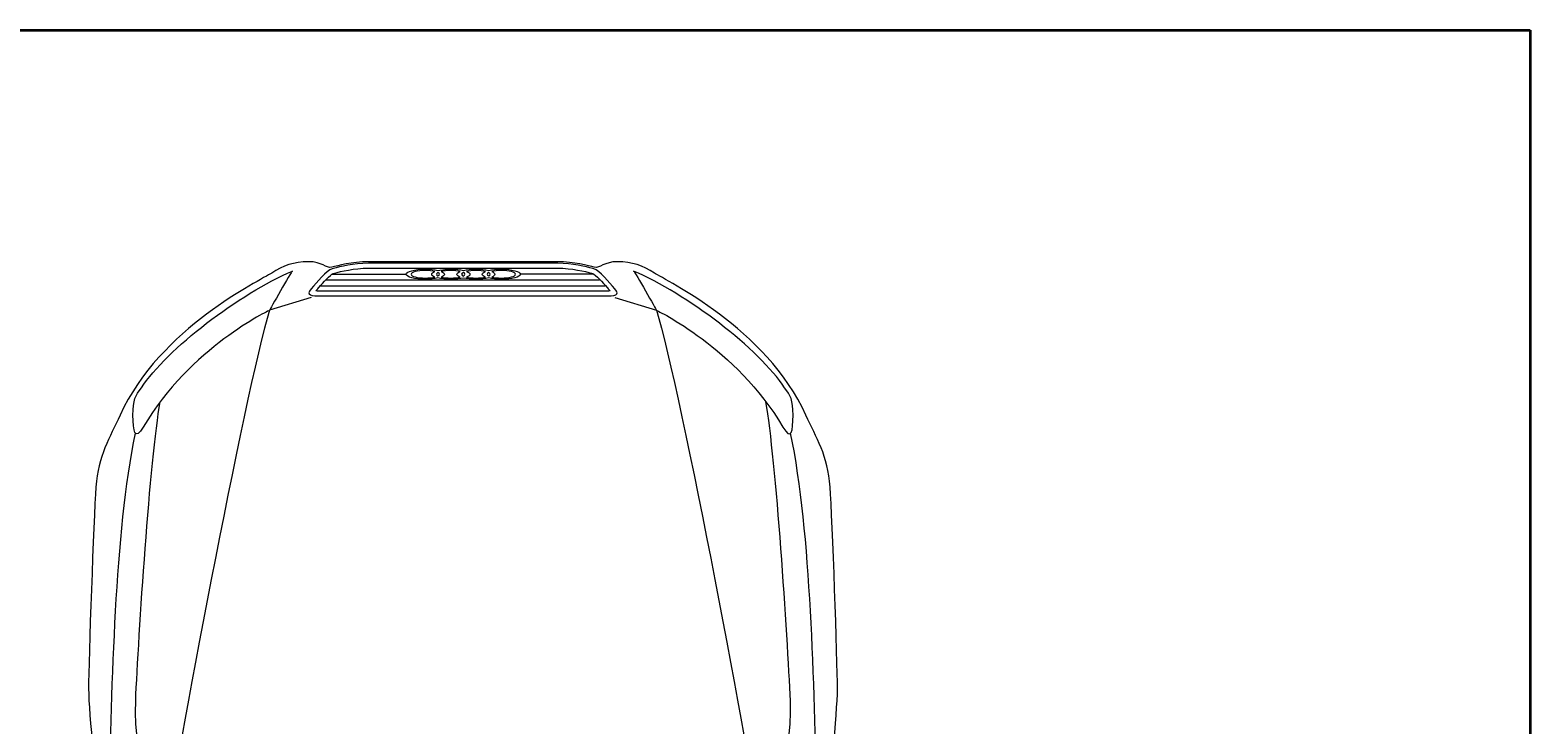
# Model space of a CAD drawing. Units: inches. Extents: x 1911 to 3278, y 2022 to 3108.
# Tile 5 of 13: x 2045 to 2118, y 2230 to 2264. Entities that reach past the tile are written whole.
import ezdxf

# ---------------------------------------------------------------- set-up
doc = ezdxf.new("R2010")
doc.units = ezdxf.units.IN
for name, color, linetype, lineweight in [('A-ANNO-DIMS', 2, 'Continuous', 18), ('A-WALL', 7, 'Continuous', 35), ('AUDI', 7, 'Continuous', 18)]:
    doc.layers.add(name, color=color, linetype=linetype, lineweight=lineweight)
doc.styles.get("Standard").update_dxf_attribs({"font": 'arial.ttf'})
doc.dimstyles.get("Standard").update_dxf_attribs({"dimtxt": 0.18, "dimasz": 0.18, "dimexe": 0.18, "dimexo": 0.0625, "dimgap": 0.09, "dimtad": 0, "dimtih": 1, "dimtoh": 1, "dimdec": 4, "dimzin": 0, "dimdsep": 46, "dimtxsty": 'Standard', "dimcen": 0.09, "dimadec": 0, "dimazin": 0, "dimtfac": 1, "dimtdec": 4, "dimtofl": 0, "dimtmove": 0, "dimatfit": 3, "dimfxl": 1, "dimtolj": 1, "dimtzin": 0, "dimarcsym": 0})

# ---------------------------------------------------------------- blocks, each defined once
blk = doc.blocks.new('*D68')
at = {"layer": 'A-ANNO-DIMS', "color": 0, "lineweight": -2, "transparency": 16777216}
for p, q in [((2016.834, 2263.811), (2016.834, 2048.124)), ((2117.834, 2263.811), (2117.834, 2048.124)), ((2017.014, 2048.304), (2067.071, 2048.304)), ((2117.654, 2048.304), (2067.597, 2048.304))]:
    blk.add_line(p, q, dxfattribs=at)
at = {"layer": 'A-ANNO-DIMS', "color": 0, "transparency": 16777216}
for points in [[(2017.014, 2048.334), (2017.014, 2048.274), (2016.834, 2048.304)], [(2117.654, 2048.334), (2117.654, 2048.274), (2117.834, 2048.304)]]:
    blk.add_solid(points, dxfattribs=at)
at = {"layer": 'Defpoints', "color": 0, "transparency": 16777216}
for p in [(2016.834, 2263.873), (2117.834, 2263.873), (2117.834, 2048.304)]:
    blk.add_point(p, dxfattribs=at)
at = {"layer": 'A-ANNO-DIMS', "color": 0, "transparency": 16777216, "insert": (2067.334, 2048.304), "char_height": 0.18, "attachment_point": 5}
blk.add_mtext('\\A1;101', dxfattribs=at)

msp = doc.modelspace()

# ---------------------------------------------------------------- linework, layer by layer
at = {"layer": 'A-WALL'}
for p, q in [((2016.8344, 2263.8733), (2117.8344, 2263.8733)), ((2117.8344, 2263.8733), (2117.8344, 2217.8733))]:
    msp.add_line(p, q, dxfattribs=at)
at = {"layer": 'AUDI'}
for points, knots in [([(2065.7636, 2161.2036), (2052.3657, 2161.35), (2050.4204, 2165.8553), (2049.5983, 2168.8238), (2049.5983, 2168.8238), (2049.0621, 2170.5764), (2048.6333, 2171.9712), (2048.4187, 2172.6866), (2048.4187, 2172.6866), (2048.2042, 2173.4019), (2047.7397, 2175.5836), (2047.7038, 2177.4077), (2047.7038, 2177.4077), (2047.6679, 2179.2318), (2047.491, 2190.1075), (2047.491, 2193.1091), (2047.491, 2193.1091), (2047.491, 2196.1105), (2047.491, 2210.1722), (2047.491, 2212.1725), (2047.491, 2212.1725), (2047.491, 2214.1727), (2047.9184, 2222.1512), (2047.9184, 2224.6905), (2047.9184, 2224.6905), (2047.9184, 2227.23), (2047.491, 2230.416), (2047.491, 2231.7362), (2047.491, 2231.7362), (2047.491, 2233.0566), (2047.7395, 2240.034), (2047.8468, 2241.572), (2047.8468, 2241.572), (2047.9542, 2243.11), (2048.5301, 2243.9822), (2049.0266, 2245.0771), (2049.0266, 2245.0771), (2050.9569, 2249.333), (2055.8898, 2251.6577), (2056.426, 2252.0154), (2056.426, 2252.0154), (2056.9622, 2252.3732), (2057.5315, 2252.5675), (2058.2133, 2252.5675), (2058.2133, 2252.5675), (2058.8952, 2252.5675), (2059.0712, 2252.2302), (2059.3573, 2252.3017), (2059.3573, 2252.3017), (2059.6432, 2252.3732), (2060.3558, 2252.5675), (2061.1448, 2252.5675), (2061.1448, 2252.5675), (2061.9338, 2252.5675), (2065.7636, 2252.5675), (2065.7636, 2252.5675), (2065.7636, 2252.5675), (2065.7636, 2252.5675), (2069.5936, 2252.5675), (2070.3825, 2252.5675), (2070.3825, 2252.5675), (2071.1717, 2252.5675), (2071.8841, 2252.3732), (2072.1701, 2252.3017), (2072.1701, 2252.3017), (2072.4561, 2252.2302), (2072.6322, 2252.5675), (2073.314, 2252.5675), (2073.314, 2252.5675), (2073.9959, 2252.5675), (2074.5651, 2252.3732), (2075.1013, 2252.0154), (2075.1013, 2252.0154), (2075.6375, 2251.6577), (2080.5704, 2249.333), (2082.5007, 2245.0771), (2082.5007, 2245.0771), (2082.9972, 2243.9822), (2083.5731, 2243.1099), (2083.6805, 2241.572), (2083.6805, 2241.572), (2083.7879, 2240.0341), (2084.0364, 2233.0565), (2084.0364, 2231.7362), (2084.0364, 2231.7362), (2084.0364, 2230.4161), (2083.609, 2227.23), (2083.609, 2224.6905), (2083.609, 2224.6905), (2083.609, 2222.1512), (2084.0364, 2214.1727), (2084.0364, 2212.1725), (2084.0364, 2212.1725), (2084.0364, 2210.1722), (2084.0364, 2196.1105), (2084.0364, 2193.1091), (2084.0364, 2193.1091), (2084.0364, 2190.1075), (2083.8594, 2179.2318), (2083.8235, 2177.4077), (2083.8235, 2177.4077), (2083.7877, 2175.5836), (2083.3232, 2173.4019), (2083.1086, 2172.6866), (2083.1086, 2172.6866), (2082.8941, 2171.9712), (2082.4652, 2170.5764), (2081.9291, 2168.8238), (2081.9291, 2168.8238), (2081.107, 2165.8553), (2079.1616, 2161.35), (2065.7636, 2161.2036)], [0, 0, 0, 0, 0.0357143, 0.0357143, 0.0357143, 0.0357143, 0.0714286, 0.0714286, 0.0714286, 0.0714286, 0.1071429, 0.1071429, 0.1071429, 0.1071429, 0.1428571, 0.1428571, 0.1428571, 0.1428572, 0.1785714, 0.1785714, 0.1785714, 0.1785714, 0.2142857, 0.2142857, 0.2142857, 0.2142857, 0.25, 0.25, 0.25, 0.25, 0.2857143, 0.2857143, 0.2857143, 0.2857143, 0.3214286, 0.3214286, 0.3214286, 0.3214286, 0.3571429, 0.3571429, 0.3571429, 0.3571429, 0.3928571, 0.3928571, 0.3928571, 0.3928572, 0.4285714, 0.4285714, 0.4285714, 0.4285714, 0.4642857, 0.4642857, 0.4642857, 0.4642857, 0.5, 0.5, 0.5, 0.5, 0.5357143, 0.5357143, 0.5357143, 0.5357143, 0.5714286, 0.5714286, 0.5714286, 0.5714286, 0.6071429, 0.6071429, 0.6071429, 0.6071429, 0.6428571, 0.6428571, 0.6428571, 0.6428572, 0.6785714, 0.6785714, 0.6785714, 0.6785714, 0.7142857, 0.7142857, 0.7142857, 0.7142857, 0.75, 0.75, 0.75, 0.75, 0.7857143, 0.7857143, 0.7857143, 0.7857143, 0.8214286, 0.8214286, 0.8214286, 0.8214286, 0.8571429, 0.8571429, 0.8571429, 0.8571429, 0.8928571, 0.8928571, 0.8928571, 0.8928572, 0.9285714, 0.9285714, 0.9285714, 0.9285714, 0.9642857, 0.9642857, 0.9642857, 0.9642857, 1, 1, 1, 1]), ([(2065.8389, 2252.4894), (2065.8389, 2252.4894), (2070.3825, 2252.4894), (2070.3825, 2252.4894), (2070.3825, 2252.4894), (2071.1113, 2252.4894), (2071.7728, 2252.3216), (2072.0906, 2252.2412), (2072.0906, 2252.2412), (2072.0906, 2252.2412), (2072.1511, 2252.2259), (2072.1511, 2252.2259), (2072.1511, 2252.2259), (2072.44, 2252.1337), (2072.887, 2251.5522), (2073.1702, 2251.2391), (2073.1702, 2251.2391), (2073.4534, 2250.9259), (2073.1702, 2250.8962), (2072.6635, 2250.8962), (2072.6635, 2250.8962), (2072.1568, 2250.8962), (2065.7636, 2250.8962), (2065.7636, 2250.8962), (2065.7636, 2250.8962), (2065.7636, 2250.8962), (2059.3705, 2250.8962), (2058.8638, 2250.8962), (2058.8638, 2250.8962), (2058.3572, 2250.8962), (2058.074, 2250.9259), (2058.3572, 2251.2391), (2058.3572, 2251.2391), (2058.6403, 2251.5522), (2059.0873, 2252.1336), (2059.3762, 2252.2259), (2059.3762, 2252.2259), (2059.3762, 2252.2259), (2059.4367, 2252.2412), (2059.4367, 2252.2412), (2059.4367, 2252.2412), (2059.7545, 2252.3216), (2060.416, 2252.4893), (2061.1448, 2252.4893), (2061.1448, 2252.4893), (2061.1448, 2252.4893), (2065.6885, 2252.4894), (2065.6885, 2252.4894), (2065.6885, 2252.4894), (2065.6885, 2252.4894), (2065.8389, 2252.4894), (2065.8389, 2252.4894)], [0, 0, 0, 0, 0.0769231, 0.0769231, 0.0769231, 0.0769231, 0.1538462, 0.1538462, 0.1538462, 0.1538462, 0.2307692, 0.2307692, 0.2307692, 0.2307692, 0.3076923, 0.3076923, 0.3076923, 0.3076923, 0.3846154, 0.3846154, 0.3846154, 0.3846154, 0.4615385, 0.4615385, 0.4615385, 0.4615385, 0.5384615, 0.5384615, 0.5384615, 0.5384615, 0.6153846, 0.6153846, 0.6153846, 0.6153846, 0.6923077, 0.6923077, 0.6923077, 0.6923077, 0.7692308, 0.7692308, 0.7692308, 0.7692308, 0.8461538, 0.8461538, 0.8461538, 0.8461539, 0.9230769, 0.9230769, 0.9230769, 0.9230769, 1, 1, 1, 1]), ([(2049.6568, 2245.0859), (2049.6568, 2244.2903), (2049.748, 2243.8077), (2050.1559, 2244.4983), (2050.1559, 2244.4983), (2052.4466, 2248.3769), (2056.3231, 2250.1984), (2056.3231, 2250.1984), (2056.3231, 2250.1984), (2056.3231, 2250.1984), (2057.3734, 2252.0821), (2057.4391, 2252.1083), (2057.4391, 2252.1083), (2054.8815, 2251.0258), (2051.2895, 2248.298), (2050.0679, 2246.4083), (2050.0679, 2246.4083), (2049.7743, 2246.0263), (2049.6568, 2245.8358), (2049.6568, 2245.0859)], [0, 0, 0, 0, 0.2, 0.2, 0.2, 0.2, 0.4, 0.4, 0.4, 0.4, 0.6, 0.6, 0.6, 0.6, 0.8, 0.8, 0.8, 0.8, 1, 1, 1, 1]), ([(2049.6568, 2245.0859), (2049.6568, 2244.2903), (2049.748, 2243.8077), (2050.1559, 2244.4983), (2050.1559, 2244.4983), (2052.4466, 2248.3769), (2056.3231, 2250.1984), (2056.3231, 2250.1984), (2056.3231, 2250.1984), (2056.3231, 2250.1984), (2057.3734, 2252.0821), (2057.4391, 2252.1083), (2057.4391, 2252.1083), (2054.8815, 2251.0258), (2051.2895, 2248.298), (2050.0679, 2246.4083), (2050.0679, 2246.4083), (2049.7743, 2246.0263), (2049.6568, 2245.8358), (2049.6568, 2245.0859)], [0, 0, 0, 0, 0.2, 0.2, 0.2, 0.2, 0.4, 0.4, 0.4, 0.4, 0.6, 0.6, 0.6, 0.6, 0.8, 0.8, 0.8, 0.8, 1, 1, 1, 1]), ([(2058.8638, 2251.1329), (2058.8638, 2251.1329), (2058.8638, 2251.1329), (2058.8638, 2251.1329), (2058.8638, 2251.1329), (2058.8638, 2251.1329), (2072.6635, 2251.1329), (2072.6635, 2251.1329), (2072.6635, 2251.1329), (2072.78, 2251.1329), (2072.8697, 2251.1357), (2072.9424, 2251.1402), (2072.9424, 2251.1402), (2072.8866, 2251.2042), (2072.8004, 2251.3028), (2072.8004, 2251.3028), (2072.8004, 2251.3028), (2072.593, 2251.5439), (2072.2461, 2251.9466), (2072.0796, 2252), (2072.0796, 2252), (2072.0796, 2252), (2072.0328, 2252.0116), (2072.0328, 2252.0116), (2072.0328, 2252.0116), (2071.7231, 2252.0901), (2071.0812, 2252.2528), (2070.3825, 2252.2528), (2070.3825, 2252.2528), (2070.3825, 2252.2528), (2061.1448, 2252.2528), (2061.1448, 2252.2528), (2061.1448, 2252.2528), (2060.4462, 2252.2528), (2059.8043, 2252.09), (2059.4956, 2252.012), (2059.4956, 2252.012), (2059.4956, 2252.012), (2059.4341, 2251.9963), (2059.4341, 2251.9963), (2059.4341, 2251.9963), (2059.2817, 2251.9474), (2058.9346, 2251.5438), (2058.7269, 2251.3028), (2058.7269, 2251.3028), (2058.7269, 2251.3028), (2058.641, 2251.2042), (2058.585, 2251.1402), (2058.585, 2251.1402), (2058.6579, 2251.1358), (2058.7473, 2251.1329), (2058.8638, 2251.1329)], [0, 0, 0, 0, 0.0769231, 0.0769231, 0.0769231, 0.0769231, 0.1538462, 0.1538462, 0.1538462, 0.1538462, 0.2307692, 0.2307692, 0.2307692, 0.2307692, 0.3076923, 0.3076923, 0.3076923, 0.3076923, 0.3846154, 0.3846154, 0.3846154, 0.3846154, 0.4615385, 0.4615385, 0.4615385, 0.4615385, 0.5384615, 0.5384615, 0.5384615, 0.5384615, 0.6153846, 0.6153846, 0.6153846, 0.6153846, 0.6923077, 0.6923077, 0.6923077, 0.6923077, 0.7692308, 0.7692308, 0.7692308, 0.7692308, 0.8461538, 0.8461538, 0.8461538, 0.8461539, 0.9230769, 0.9230769, 0.9230769, 0.9230769, 1, 1, 1, 1]), ([(2063.921, 2251.7091), (2064.1614, 2251.7091), (2064.3716, 2251.7333), (2064.5366, 2251.7741), (2064.5366, 2251.7741), (2064.702, 2251.7333), (2064.9274, 2251.7091), (2065.1678, 2251.7091), (2065.1678, 2251.7091), (2065.4079, 2251.7091), (2065.6182, 2251.7333), (2065.7835, 2251.77), (2065.7835, 2251.77), (2065.9334, 2251.7333), (2066.1591, 2251.7091), (2066.3842, 2251.7091), (2066.3842, 2251.7091), (2066.6247, 2251.7091), (2066.85, 2251.7333), (2067.0152, 2251.7741), (2067.0152, 2251.7741), (2067.1804, 2251.7333), (2067.3906, 2251.7091), (2067.6309, 2251.7091), (2067.6309, 2251.7091), (2068.1418, 2251.7091), (2068.5623, 2251.8185), (2068.5623, 2251.956), (2068.5623, 2251.956), (2068.5623, 2252.0894), (2068.1418, 2252.2031), (2067.6309, 2252.2031), (2067.6309, 2252.2031), (2067.3906, 2252.2031), (2067.1804, 2252.1748), (2067.0152, 2252.1381), (2067.0152, 2252.1381), (2066.85, 2252.1748), (2066.6247, 2252.2031), (2066.3842, 2252.2031), (2066.3842, 2252.2031), (2066.1591, 2252.2031), (2065.9334, 2252.1788), (2065.7835, 2252.1381), (2065.7835, 2252.1381), (2065.6182, 2252.1789), (2065.4079, 2252.2031), (2065.1678, 2252.2031), (2065.1678, 2252.2031), (2064.9001, 2252.2031), (2064.6104, 2252.1546), (2064.5366, 2252.1381), (2064.5366, 2252.1381), (2064.3716, 2252.1748), (2064.1614, 2252.2031), (2063.921, 2252.2031), (2063.921, 2252.2031), (2063.4102, 2252.2031), (2062.9895, 2252.0894), (2062.9895, 2251.956), (2062.9895, 2251.956), (2062.9895, 2251.8185), (2063.4102, 2251.7091), (2063.921, 2251.7091)], [0, 0, 0, 0, 0.0625, 0.0625, 0.0625, 0.0625, 0.125, 0.125, 0.125, 0.125, 0.1875, 0.1875, 0.1875, 0.1875, 0.25, 0.25, 0.25, 0.25, 0.3125, 0.3125, 0.3125, 0.3125, 0.375, 0.375, 0.375, 0.375, 0.4375, 0.4375, 0.4375, 0.4375, 0.5, 0.5, 0.5, 0.5, 0.5625, 0.5625, 0.5625, 0.5625, 0.625, 0.625, 0.625, 0.625, 0.6875, 0.6875, 0.6875, 0.6875, 0.75, 0.75, 0.75, 0.75, 0.8125, 0.8125, 0.8125, 0.8125, 0.875, 0.875, 0.875, 0.875, 0.9375, 0.9375, 0.9375, 0.9375, 1, 1, 1, 1]), ([(2063.921, 2251.7091), (2064.1614, 2251.7091), (2064.3716, 2251.7333), (2064.5366, 2251.7741), (2064.5366, 2251.7741), (2064.702, 2251.7333), (2064.9274, 2251.7091), (2065.1678, 2251.7091), (2065.1678, 2251.7091), (2065.4079, 2251.7091), (2065.6182, 2251.7333), (2065.7835, 2251.77), (2065.7835, 2251.77), (2065.9334, 2251.7333), (2066.1591, 2251.7091), (2066.3842, 2251.7091), (2066.3842, 2251.7091), (2066.6247, 2251.7091), (2066.85, 2251.7333), (2067.0152, 2251.7741), (2067.0152, 2251.7741), (2067.1804, 2251.7333), (2067.3906, 2251.7091), (2067.6309, 2251.7091), (2067.6309, 2251.7091), (2068.1418, 2251.7091), (2068.5623, 2251.8185), (2068.5623, 2251.956), (2068.5623, 2251.956), (2068.5623, 2252.0894), (2068.1418, 2252.2031), (2067.6309, 2252.2031), (2067.6309, 2252.2031), (2067.3906, 2252.2031), (2067.1804, 2252.1748), (2067.0152, 2252.1381), (2067.0152, 2252.1381), (2066.85, 2252.1748), (2066.6247, 2252.2031), (2066.3842, 2252.2031), (2066.3842, 2252.2031), (2066.1591, 2252.2031), (2065.9334, 2252.1788), (2065.7835, 2252.1381), (2065.7835, 2252.1381), (2065.6182, 2252.1789), (2065.4079, 2252.2031), (2065.1678, 2252.2031), (2065.1678, 2252.2031), (2064.9001, 2252.2031), (2064.6104, 2252.1546), (2064.5366, 2252.1381), (2064.5366, 2252.1381), (2064.3716, 2252.1748), (2064.1614, 2252.2031), (2063.921, 2252.2031), (2063.921, 2252.2031), (2063.4102, 2252.2031), (2062.9895, 2252.0894), (2062.9895, 2251.956), (2062.9895, 2251.956), (2062.9895, 2251.8185), (2063.4102, 2251.7091), (2063.921, 2251.7091)], [0, 0, 0, 0, 0.0625, 0.0625, 0.0625, 0.0625, 0.125, 0.125, 0.125, 0.125, 0.1875, 0.1875, 0.1875, 0.1875, 0.25, 0.25, 0.25, 0.25, 0.3125, 0.3125, 0.3125, 0.3125, 0.375, 0.375, 0.375, 0.375, 0.4375, 0.4375, 0.4375, 0.4375, 0.5, 0.5, 0.5, 0.5, 0.5625, 0.5625, 0.5625, 0.5625, 0.625, 0.625, 0.625, 0.625, 0.6875, 0.6875, 0.6875, 0.6875, 0.75, 0.75, 0.75, 0.75, 0.8125, 0.8125, 0.8125, 0.8125, 0.875, 0.875, 0.875, 0.875, 0.9375, 0.9375, 0.9375, 0.9375, 1, 1, 1, 1]), ([(2063.921, 2252.1381), (2064.1011, 2252.1381), (2064.2665, 2252.122), (2064.3867, 2252.0894), (2064.3867, 2252.0894), (2064.2964, 2252.0491), (2064.2363, 2252.0046), (2064.2363, 2251.956), (2064.2363, 2251.956), (2064.2363, 2251.9034), (2064.2964, 2251.859), (2064.3867, 2251.8185), (2064.3867, 2251.8185), (2064.2665, 2251.7901), (2064.1011, 2251.77), (2063.921, 2251.77), (2063.921, 2251.77), (2063.5304, 2251.77), (2063.2299, 2251.8508), (2063.2299, 2251.956), (2063.2299, 2251.956), (2063.2299, 2252.0572), (2063.5304, 2252.1381), (2063.921, 2252.1381)], [0, 0, 0, 0, 0.1666667, 0.1666667, 0.1666667, 0.1666667, 0.3333333, 0.3333333, 0.3333333, 0.3333333, 0.5, 0.5, 0.5, 0.5, 0.6666667, 0.6666667, 0.6666667, 0.6666667, 0.8333333, 0.8333333, 0.8333333, 0.8333333, 1, 1, 1, 1]), ([(2064.612, 2251.956), (2064.612, 2251.9236), (2064.5819, 2251.8993), (2064.5366, 2251.8751), (2064.5366, 2251.8751), (2064.4918, 2251.8994), (2064.4767, 2251.9235), (2064.4767, 2251.956), (2064.4767, 2251.956), (2064.4767, 2251.9845), (2064.4918, 2252.0126), (2064.5366, 2252.037), (2064.5366, 2252.037), (2064.5819, 2252.0126), (2064.612, 2251.9845), (2064.612, 2251.956)], [0, 0, 0, 0, 0.25, 0.25, 0.25, 0.25, 0.5, 0.5, 0.5, 0.5, 0.75, 0.75, 0.75, 0.75, 1, 1, 1, 1]), ([(2065.6182, 2252.0935), (2065.5279, 2252.0532), (2065.4681, 2252.0046), (2065.4681, 2251.956), (2065.4681, 2251.956), (2065.4681, 2251.9034), (2065.5279, 2251.8549), (2065.6182, 2251.8144), (2065.6182, 2251.8144), (2065.4982, 2251.7861), (2065.3479, 2251.77), (2065.1678, 2251.77), (2065.1678, 2251.77), (2064.9873, 2251.77), (2064.8223, 2251.7901), (2064.702, 2251.8185), (2064.702, 2251.8185), (2064.7921, 2251.859), (2064.8522, 2251.9034), (2064.8522, 2251.956), (2064.8522, 2251.956), (2064.8522, 2252.0047), (2064.7921, 2252.0491), (2064.702, 2252.0894), (2064.702, 2252.0894), (2064.8223, 2252.1221), (2064.9873, 2252.1381), (2065.1678, 2252.1381), (2065.1678, 2252.1381), (2065.3479, 2252.1381), (2065.4982, 2252.122), (2065.6182, 2252.0935)], [0, 0, 0, 0, 0.125, 0.125, 0.125, 0.125, 0.25, 0.25, 0.25, 0.25, 0.375, 0.375, 0.375, 0.375, 0.5, 0.5, 0.5, 0.5, 0.625, 0.625, 0.625, 0.625, 0.75, 0.75, 0.75, 0.75, 0.875, 0.875, 0.875, 0.875, 1, 1, 1, 1]), ([(2065.8584, 2251.956), (2065.8584, 2251.9236), (2065.8286, 2251.8952), (2065.7835, 2251.8669), (2065.7835, 2251.8669), (2065.7233, 2251.8953), (2065.6934, 2251.9235), (2065.6934, 2251.956), (2065.6934, 2251.956), (2065.6934, 2251.9845), (2065.7233, 2252.0167), (2065.7835, 2252.0411), (2065.7835, 2252.0411), (2065.8286, 2252.0167), (2065.8584, 2251.9845), (2065.8584, 2251.956)], [0, 0, 0, 0, 0.25, 0.25, 0.25, 0.25, 0.5, 0.5, 0.5, 0.5, 0.75, 0.75, 0.75, 0.75, 1, 1, 1, 1]), ([(2066.8648, 2252.0894), (2066.7597, 2252.0491), (2066.6998, 2252.0046), (2066.6998, 2251.956), (2066.6998, 2251.956), (2066.6998, 2251.9034), (2066.7597, 2251.859), (2066.8648, 2251.8185), (2066.8648, 2251.8185), (2066.7297, 2251.7901), (2066.5645, 2251.77), (2066.3842, 2251.77), (2066.3842, 2251.77), (2066.219, 2251.77), (2066.0538, 2251.7861), (2065.9334, 2251.8144), (2065.9334, 2251.8144), (2066.0389, 2251.855), (2066.0988, 2251.9034), (2066.0988, 2251.956), (2066.0988, 2251.956), (2066.0988, 2252.0047), (2066.0389, 2252.0531), (2065.9334, 2252.0934), (2065.9334, 2252.0934), (2066.0538, 2252.1221), (2066.219, 2252.1381), (2066.3842, 2252.1381), (2066.3842, 2252.1381), (2066.5645, 2252.1381), (2066.7297, 2252.122), (2066.8648, 2252.0894)], [0, 0, 0, 0, 0.125, 0.125, 0.125, 0.125, 0.25, 0.25, 0.25, 0.25, 0.375, 0.375, 0.375, 0.375, 0.5, 0.5, 0.5, 0.5, 0.625, 0.625, 0.625, 0.625, 0.75, 0.75, 0.75, 0.75, 0.875, 0.875, 0.875, 0.875, 1, 1, 1, 1]), ([(2067.0901, 2251.956), (2067.0901, 2251.9236), (2067.0602, 2251.8993), (2067.0152, 2251.8751), (2067.0152, 2251.8751), (2066.97, 2251.8994), (2066.94, 2251.9235), (2066.94, 2251.956), (2066.94, 2251.956), (2066.94, 2251.9845), (2066.97, 2252.0126), (2067.0152, 2252.037), (2067.0152, 2252.037), (2067.0602, 2252.0126), (2067.0901, 2251.9845), (2067.0901, 2251.956)], [0, 0, 0, 0, 0.25, 0.25, 0.25, 0.25, 0.5, 0.5, 0.5, 0.5, 0.75, 0.75, 0.75, 0.75, 1, 1, 1, 1]), ([(2068.3219, 2251.956), (2068.3219, 2251.8509), (2068.0216, 2251.77), (2067.6309, 2251.77), (2067.6309, 2251.77), (2067.4507, 2251.77), (2067.2855, 2251.7901), (2067.1653, 2251.8185), (2067.1653, 2251.8185), (2067.2556, 2251.859), (2067.3155, 2251.9034), (2067.3155, 2251.956), (2067.3155, 2251.956), (2067.3155, 2252.0047), (2067.2556, 2252.0491), (2067.1653, 2252.0894), (2067.1653, 2252.0894), (2067.2855, 2252.1221), (2067.4507, 2252.1381), (2067.6309, 2252.1381), (2067.6309, 2252.1381), (2068.0216, 2252.1381), (2068.3219, 2252.0572), (2068.3219, 2251.956)], [0, 0, 0, 0, 0.1666667, 0.1666667, 0.1666667, 0.1666667, 0.3333333, 0.3333333, 0.3333333, 0.3333333, 0.5, 0.5, 0.5, 0.5, 0.6666667, 0.6666667, 0.6666667, 0.6666667, 0.8333333, 0.8333333, 0.8333333, 0.8333333, 1, 1, 1, 1]), ([(2081.8706, 2245.0859), (2081.8706, 2244.2903), (2081.7793, 2243.8077), (2081.3715, 2244.4983), (2081.3715, 2244.4983), (2079.0807, 2248.3769), (2075.2042, 2250.1984), (2075.2042, 2250.1984), (2075.2042, 2250.1984), (2075.2042, 2250.1984), (2074.154, 2252.0821), (2074.0882, 2252.1083), (2074.0882, 2252.1083), (2076.6458, 2251.0258), (2080.2379, 2248.298), (2081.4595, 2246.4083), (2081.4595, 2246.4083), (2081.753, 2246.0263), (2081.8706, 2245.8358), (2081.8706, 2245.0859)], [0, 0, 0, 0, 0.2, 0.2, 0.2, 0.2, 0.4, 0.4, 0.4, 0.4, 0.6, 0.6, 0.6, 0.6, 0.8, 0.8, 0.8, 0.8, 1, 1, 1, 1]), ([(2081.8706, 2245.0859), (2081.8706, 2244.2903), (2081.7793, 2243.8077), (2081.3715, 2244.4983), (2081.3715, 2244.4983), (2079.0807, 2248.3769), (2075.2042, 2250.1984), (2075.2042, 2250.1984), (2075.2042, 2250.1984), (2075.2042, 2250.1984), (2074.154, 2252.0821), (2074.0882, 2252.1083), (2074.0882, 2252.1083), (2076.6458, 2251.0258), (2080.2379, 2248.298), (2081.4595, 2246.4083), (2081.4595, 2246.4083), (2081.753, 2246.0263), (2081.8706, 2245.8358), (2081.8706, 2245.0859)], [0, 0, 0, 0, 0.2, 0.2, 0.2, 0.2, 0.4, 0.4, 0.4, 0.4, 0.6, 0.6, 0.6, 0.6, 0.8, 0.8, 0.8, 0.8, 1, 1, 1, 1]), ([(2051.3626, 2225.4871), (2050.9454, 2226.322), (2049.6509, 2227.988), (2049.7888, 2231.1364), (2049.7888, 2231.1364), (2049.9267, 2234.2849), (2050.4858, 2242.9716), (2050.9873, 2245.7351)], [0, 0, 0, 0, 0.5, 0.5, 0.5, 0.5, 1, 1, 1, 1]), ([(2080.1647, 2225.4871), (2080.582, 2226.322), (2081.8765, 2227.988), (2081.7386, 2231.1364), (2081.7386, 2231.1364), (2081.6006, 2234.2849), (2081.0416, 2242.9716), (2080.54, 2245.7351)], [0, 0, 0, 0, 0.5, 0.5, 0.5, 0.5, 1, 1, 1, 1]), ([(2050.2266, 2168.7846), (2049.5535, 2172.1525), (2048.8368, 2178.9728), (2048.7144, 2186.0758), (2048.7144, 2186.0758), (2048.5919, 2193.1787), (2048.2861, 2220.4882), (2048.4696, 2226.2439), (2048.4696, 2226.2439), (2048.6532, 2231.9997), (2048.7559, 2239.2607), (2049.7755, 2244.2027)], [0, 0, 0, 0, 0.3333333, 0.3333333, 0.3333333, 0.3333333, 0.6666667, 0.6666667, 0.6666667, 0.6666667, 1, 1, 1, 1]), ([(2081.3007, 2168.7846), (2081.9739, 2172.1525), (2082.6906, 2178.9728), (2082.813, 2186.0758), (2082.813, 2186.0758), (2082.9355, 2193.1787), (2083.2413, 2220.4882), (2083.0577, 2226.2439), (2083.0577, 2226.2439), (2082.8742, 2231.9997), (2082.7714, 2239.2607), (2081.7518, 2244.2027)], [0, 0, 0, 0, 0.3333333, 0.3333333, 0.3333333, 0.3333333, 0.6666667, 0.6666667, 0.6666667, 0.6666667, 1, 1, 1, 1])]:
    msp.add_open_spline(points, degree=3, knots=knots, dxfattribs=at)
for points in [[(2059.376, 2251.9664), (2059.376, 2251.9664), (2062.9895, 2251.9664), (2062.9895, 2251.9664)], [(2072.1513, 2251.9664), (2072.1513, 2251.9664), (2068.5378, 2251.9664), (2068.5378, 2251.9664)], [(2058.8035, 2251.3917), (2058.8035, 2251.3917), (2072.7075, 2251.3917), (2072.7075, 2251.3917)], [(2059.0671, 2251.6852), (2059.0671, 2251.6852), (2072.4215, 2251.6852), (2072.4215, 2251.6852)], [(2058.3524, 2250.822), (2058.3524, 2250.822), (2056.3231, 2250.1984), (2056.3231, 2250.1984)], [(2073.1749, 2250.822), (2073.1749, 2250.822), (2075.2042, 2250.1984), (2075.2042, 2250.1984)], [(2056.3231, 2250.1984), (2055.1434, 2246.4433), (2051.5649, 2227.2055), (2051.3563, 2225.3269)], [(2075.2042, 2250.1984), (2076.384, 2246.4433), (2079.9624, 2227.2055), (2080.1711, 2225.3269)]]:
    msp.add_open_spline(points, degree=3, dxfattribs=at)

# ---------------------------------------------------------------- dimensions: what is measured, and where the dimension line sits
at = {"layer": 'A-ANNO-DIMS'}
dim = msp.add_linear_dim(base=(2117.8344, 2048.3043), p1=(2016.8344, 2263.8733), p2=(2117.8344, 2263.8733), dimstyle='Standard', override={"dimdec": 0, "dimlfac": 1, "dimrnd": 0, "dimzin": 0, "dimdsep": 46, "dimlunit": 2}, dxfattribs=at)
dim.commit()
dim.dimension.update_dxf_attribs({"geometry": '*D68', "text_midpoint": (2067.3344, 2048.3043)})

doc.saveas('drawing.dxf')
